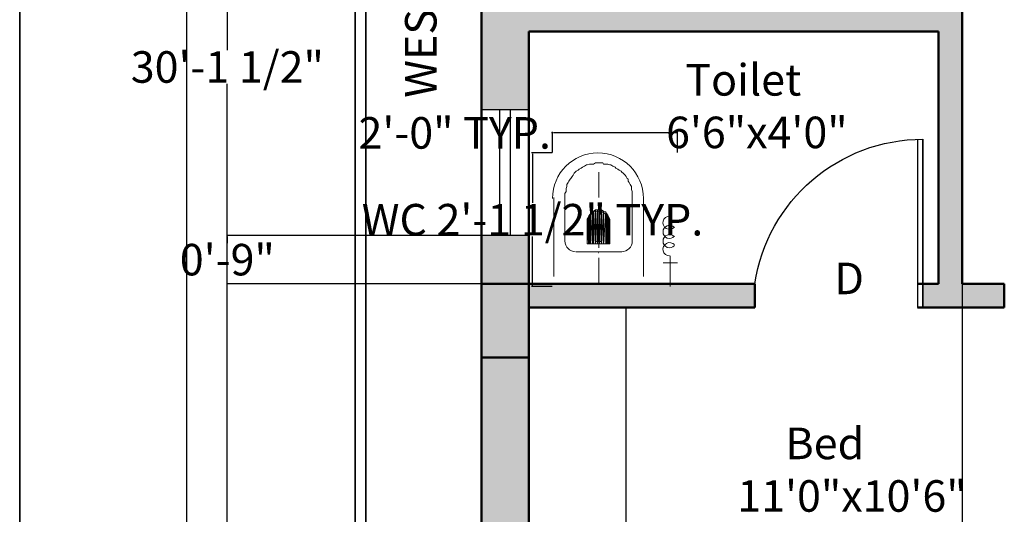
# Model space of a CAD drawing. Units: inches. Extents: x 1601 to 2080, y 5000 to 5589.
# Tile 2 of 11: x 1601 to 1788, y 5165 to 5259. Entities that reach past the tile are written whole.
import ezdxf

# ---------------------------------------------------------------- set-up
doc = ezdxf.new("R2010")
doc.units = ezdxf.units.IN
doc.header["$MEASUREMENT"] = 0
for name, color, linetype, lineweight in [('A-ANNO-DIMS', 2, 'Continuous', 18), ('A-ANNO-TEXT', 7, 'Continuous', 25), ('A-ANNO-TTLB', 7, 'Continuous', 35), ('A-AREA-IDEN', 7, 'Continuous', 25), ('A-COLS', 7, 'Continuous', 50), ('A-COLS-PATT', 18, 'Continuous', 13), ('A-DOOR', 3, 'Continuous', 25), ('A-FLOR-CASE', 8, 'Continuous', 25), ('A-FLOR-FIXT', 7, 'Continuous', 18), ('A-GLAZ', 4, 'Continuous', 25), ('A-WALL', 7, 'Continuous', 50), ('A-WALL-PATT', 241, 'Continuous', 13), ('C-PROP', 7, 'Continuous', 35)]:
    doc.layers.add(name, color=color, linetype=linetype, lineweight=lineweight)
doc.styles.get("Standard").update_dxf_attribs({"font": 'arial.ttf'})
doc.dimstyles.get("Standard").update_dxf_attribs({"dimtxt": 6, "dimasz": 0.18, "dimexe": 0.18, "dimexo": 0.0625, "dimgap": 0.09, "dimtad": 0, "dimtih": 1, "dimtoh": 1, "dimdec": 1, "dimzin": 0, "dimdsep": 46, "dimlunit": 3, "dimtxsty": 'Standard', "dimcen": 0.09, "dimadec": 0, "dimazin": 0, "dimtfac": 1, "dimtdec": 1, "dimtofl": 0, "dimtmove": 0, "dimatfit": 3, "dimfxl": 1, "dimtolj": 1, "dimtzin": 0, "dimarcsym": 0})

# ---------------------------------------------------------------- blocks, each defined once
blk = doc.blocks.new('*D4')
at = {"layer": 'A-ANNO-DIMS', "color": 0, "lineweight": -2, "transparency": 16777216}
for p, q in [((1664.35, 5509.2), (1632.18, 5509.2)), ((1632.36, 5509.02), (1632.36, 5281.35)), ((1632.36, 5047.39), (1632.36, 5275.05)), ((1664.35, 5047.21), (1632.18, 5047.21))]:
    blk.add_line(p, q, dxfattribs=at)
at = {"layer": 'A-ANNO-DIMS', "color": 0, "transparency": 16777216}
for points in [[(1632.33, 5509.02), (1632.39, 5509.02), (1632.36, 5509.2)], [(1632.33, 5047.39), (1632.39, 5047.39), (1632.36, 5047.21)]]:
    blk.add_solid(points, dxfattribs=at)
at = {"layer": 'Defpoints', "color": 0, "transparency": 16777216}
for p in [(1664.41, 5509.2), (1632.36, 5047.21), (1664.41, 5047.21)]:
    blk.add_point(p, dxfattribs=at)
at = {"layer": 'A-ANNO-DIMS', "color": 0, "transparency": 16777216, "insert": (1632.36, 5278.2), "char_height": 6, "attachment_point": 5}
blk.add_mtext("\\A1;40'", dxfattribs=at)
blk = doc.blocks.new('WC')
h = blk.add_hatch(color=256)
h.paths.add_polyline_path([(12.84, 17.3), (12.84, 12.59), (13.07, 17.3)])
h.paths.add_polyline_path([(12.84, 12.59), (13.07, 17.3), (13.07, 12.21)])
h = blk.add_hatch(color=256)
h.paths.add_polyline_path([(13.07, 17.3), (13.07, 12.21), (13.22, 17.3)])
h.paths.add_polyline_path([(13.07, 12.21), (13.22, 17.3), (13.22, 11.83)])
h = blk.add_hatch(color=256)
h.paths.add_polyline_path([(13.22, 17.3), (13.22, 11.83), (13.45, 17.3)])
h.paths.add_polyline_path([(13.22, 11.83), (13.45, 17.3), (13.45, 11.61)])
h = blk.add_hatch(color=256)
h.paths.add_polyline_path([(13.45, 17.3), (13.45, 11.61), (13.6, 17.3)])
h.paths.add_polyline_path([(13.45, 11.61), (13.6, 17.3), (13.6, 11.23)])
h = blk.add_hatch(color=256)
h.paths.add_polyline_path([(13.6, 17.3), (13.6, 11.23), (14.06, 17.3)])
h.paths.add_polyline_path([(13.6, 11.23), (14.06, 17.3), (14.06, 11.08)])
h = blk.add_hatch(color=256)
h.paths.add_polyline_path([(14.06, 17.3), (14.06, 11.08), (14.44, 17.3)])
h.paths.add_polyline_path([(14.06, 11.08), (14.44, 17.3), (14.44, 10.85)])
h = blk.add_hatch(color=256)
h.paths.add_polyline_path([(14.44, 17.3), (14.44, 10.85), (14.81, 17.3)])
h.paths.add_polyline_path([(14.44, 10.85), (14.81, 17.3), (14.81, 10.85)])
h = blk.add_hatch(color=256)
h.paths.add_polyline_path([(14.81, 17.3), (14.81, 10.85), (15.19, 17.3)])
h.paths.add_polyline_path([(14.81, 10.85), (15.19, 17.3), (15.19, 10.85)])
h = blk.add_hatch(color=256)
h.paths.add_polyline_path([(15.19, 17.3), (15.19, 10.85), (15.57, 17.3)])
h.paths.add_polyline_path([(15.19, 10.85), (15.57, 17.3), (15.57, 10.85)])
h = blk.add_hatch(color=256)
h.paths.add_polyline_path([(15.57, 17.3), (15.57, 10.85), (15.95, 17.3)])
h.paths.add_polyline_path([(15.57, 10.85), (15.95, 17.3), (15.95, 11.08)])
h = blk.add_hatch(color=256)
h.paths.add_polyline_path([(15.95, 17.3), (15.95, 11.08), (16.18, 17.3)])
h.paths.add_polyline_path([(15.95, 11.08), (16.18, 17.3), (16.18, 11.23)])
h = blk.add_hatch(color=256)
h.paths.add_polyline_path([(16.18, 17.3), (16.18, 11.23), (16.56, 17.3)])
h.paths.add_polyline_path([(16.18, 11.23), (16.56, 17.3), (16.56, 11.61)])
h = blk.add_hatch(color=256)
h.paths.add_polyline_path([(16.56, 17.3), (16.56, 11.61), (16.71, 17.3)])
h.paths.add_polyline_path([(16.56, 11.61), (16.71, 17.3), (16.71, 11.83)])
h = blk.add_hatch(color=256)
h.paths.add_polyline_path([(16.71, 17.3), (16.71, 11.83), (16.94, 17.3)])
h.paths.add_polyline_path([(16.71, 11.83), (16.94, 17.3), (16.94, 12.21)])
h = blk.add_hatch(color=256)
h.paths.add_polyline_path([(16.94, 17.3), (16.94, 12.21), (17.17, 17.3)])
h.paths.add_polyline_path([(16.94, 12.21), (17.17, 17.3), (17.17, 12.59)])
h.paths.add_polyline_path([(17.17, 17.3), (17.17, 12.59), (17.17, 12.97)])
for points in [[(1.37, 25.41), (1.37, 19.57), (1.37, 19.57)], [(14.97, 24.81), (14.97, 19.95), (14.97, 19.95)], [(6.47, 23.52), (6.47, 8.5), (6.47, 8.5)], [(23.54, 23.52), (23.54, 8.5), (23.54, 8.5)], [(2.73, 20.94), (0, 20.94), (0, 20.94)], [(19.29, 18.81), (10.57, 18.81), (10.57, 18.81)], [(14.97, 19.04), (15.04, 19.04), (15.04, 19.04)], [(17.17, 17.3), (12.84, 17.3), (12.84, 17.3)], [(12.84, 17.3), (12.84, 12.97), (12.84, 12.97)], [(14.59, 16.84), (14.59, 16.92), (14.59, 16.92)], [(14.97, 18.05), (14.97, 10.47), (14.97, 10.47)], [(14.97, 16.84), (15.04, 16.92), (15.04, 16.92)], [(15.42, 16.84), (15.42, 16.92), (15.42, 16.92)], [(17.17, 17.3), (17.17, 12.97), (17.17, 12.97)], [(8.59, 16.69), (8.59, 9.48), (8.59, 9.48)], [(14.97, 16.84), (14.81, 16.84), (14.59, 16.84)], [(15.42, 16.84), (15.19, 16.84), (14.97, 16.84)], [(21.41, 16.69), (21.41, 9.48), (21.41, 9.48)], [(21.41, 9.48), (21.41, 8.72), (21.41, 8.12), (21.41, 7.74), (21.19, 7.36), (21.19, 6.98), (21.19, 6.75), (21.03, 6.37), (21.03, 5.99), (20.81, 5.61), (20.66, 5.39), (20.43, 5.01), (20.28, 4.85), (20.05, 4.48), (19.82, 4.25), (19.67, 3.87), (19.44, 3.64), (19.29, 3.49), (18.91, 3.26), (18.68, 3.11), (18.3, 2.88), (18.08, 2.73), (17.7, 2.5), (17.32, 2.28), (17.17, 2.28), (16.71, 2.12), (16.33, 2.12), (15.95, 2.12), (15.57, 1.9), (14.97, 1.9), (14.21, 1.9), (14.06, 2.12), (13.6, 2.12), (13.22, 2.12), (12.84, 2.28), (12.69, 2.28), (12.31, 2.5), (11.86, 2.73), (11.7, 2.88), (11.32, 3.11), (11.1, 3.26), (10.72, 3.49), (10.57, 3.64), (10.34, 3.87), (9.96, 4.25), (9.73, 4.48), (9.58, 4.85), (9.35, 5.01), (9.35, 5.39), (9.2, 5.61), (8.97, 5.99), (8.75, 6.37), (8.75, 6.75), (8.75, 6.98), (8.59, 7.36), (8.59, 7.74), (8.59, 8.12), (8.59, 8.72), (8.59, 9.48)], [(14.97, 8.5), (14.97, 3.64), (14.97, 3.64)]]:
    blk.add_lwpolyline(points)
for points in [[(12.84, 17.3), (12.84, 12.97)], [(12.84, 12.97), (12.84, 17.3), (12.84, 12.59)], [(12.84, 17.3), (12.84, 12.59), (13.07, 17.3)], [(12.84, 12.59), (13.07, 17.3), (13.07, 12.21)], [(13.07, 17.3), (13.07, 12.21), (13.22, 17.3)], [(13.07, 12.21), (13.22, 17.3), (13.22, 11.83)], [(13.22, 17.3), (13.22, 11.83), (13.45, 17.3)], [(13.22, 11.83), (13.45, 17.3), (13.45, 11.61)], [(13.45, 17.3), (13.45, 11.61), (13.6, 17.3)], [(13.45, 11.61), (13.6, 17.3), (13.6, 11.23)], [(13.6, 17.3), (13.6, 11.23), (14.06, 17.3)], [(13.6, 11.23), (14.06, 17.3), (14.06, 11.08)], [(14.06, 17.3), (14.06, 11.08), (14.44, 17.3)], [(14.06, 11.08), (14.44, 17.3), (14.44, 10.85)], [(14.44, 17.3), (14.44, 10.85), (14.81, 17.3)], [(14.44, 10.85), (14.81, 17.3), (14.81, 10.85)], [(14.81, 17.3), (14.81, 10.85), (15.19, 17.3)], [(14.81, 10.85), (15.19, 17.3), (15.19, 10.85)], [(15.19, 17.3), (15.19, 10.85), (15.57, 17.3)], [(15.19, 10.85), (15.57, 17.3), (15.57, 10.85)], [(15.57, 17.3), (15.57, 10.85), (15.95, 17.3)], [(15.57, 10.85), (15.95, 17.3), (15.95, 11.08)], [(15.95, 17.3), (15.95, 11.08), (16.18, 17.3)], [(15.95, 11.08), (16.18, 17.3), (16.18, 11.23)], [(16.18, 17.3), (16.18, 11.23), (16.56, 17.3)], [(16.18, 11.23), (16.56, 17.3), (16.56, 11.61)], [(16.56, 17.3), (16.56, 11.61), (16.71, 17.3)], [(16.56, 11.61), (16.71, 17.3), (16.71, 11.83)], [(16.71, 17.3), (16.71, 11.83), (16.94, 17.3)], [(16.71, 11.83), (16.94, 17.3), (16.94, 12.21)], [(16.94, 17.3), (16.94, 12.21), (17.17, 17.3)], [(16.94, 12.21), (17.17, 17.3), (17.17, 12.59)], [(17.17, 17.3), (17.17, 12.59), (17.17, 12.97)], [(17.17, 12.59), (17.17, 17.3), (17.17, 17.3)]]:
    blk.add_lwpolyline(points, close=True)
for points, knots in [([(0.53, 17.45), (0.91, 17.07), (1.59, 16.92), (2.05, 17.22), (2.05, 17.22), (2.58, 17.52), (2.88, 18.05), (2.73, 18.66), (2.73, 18.66), (2.58, 19.19), (2.05, 19.57), (1.52, 19.57)], [0, 0, 0, 0, 0.083333, 0.083333, 0.083333, 0.083334, 0.166667, 0.166667, 0.166667, 0.166668, 1, 1, 1, 1]), ([(0.61, 15.93), (0.91, 15.55), (1.52, 15.4), (1.97, 15.63), (1.97, 15.63), (2.43, 15.78), (2.73, 16.31), (2.73, 16.76), (2.73, 16.76), (2.73, 17.3), (2.43, 17.75), (1.97, 17.98), (1.97, 17.98), (1.44, 18.13), (0.91, 17.98), (0.53, 17.6)], [0, 0, 0, 0, 0.0625, 0.0625, 0.0625, 0.062501, 0.125, 0.125, 0.125, 0.125001, 0.1875, 0.1875, 0.1875, 0.187501, 1, 1, 1, 1]), ([(0.53, 14.19), (0.91, 13.81), (1.44, 13.65), (1.97, 13.88), (1.97, 13.88), (2.43, 14.03), (2.73, 14.49), (2.73, 15.02), (2.73, 15.02), (2.73, 15.55), (2.43, 16.01), (1.97, 16.23), (1.97, 16.23), (1.44, 16.39), (0.91, 16.23), (0.53, 15.85)], [0, 0, 0, 0, 0.0625, 0.0625, 0.0625, 0.062501, 0.125, 0.125, 0.125, 0.125001, 0.1875, 0.1875, 0.1875, 0.187501, 1, 1, 1, 1]), ([(1.52, 11.99), (2.05, 11.99), (2.58, 12.44), (2.73, 12.97), (2.73, 12.97), (2.88, 13.5), (2.58, 14.11), (2.12, 14.41), (2.12, 14.41), (1.59, 14.64), (0.99, 14.56), (0.61, 14.19)], [0, 0, 0, 0, 0.083333, 0.083333, 0.083333, 0.083334, 0.166667, 0.166667, 0.166667, 0.166668, 1, 1, 1, 1]), ([(13.07, 13.12), (13.07, 11.99), (13.98, 11.08), (15.12, 11.08), (15.12, 11.08), (16.26, 11.08), (17.17, 11.99), (17.17, 13.12)], [0, 0, 0, 0, 0.125, 0.125, 0.125, 0.125001, 1, 1, 1, 1]), ([(6.47, 8.65), (6.47, 3.87), (10.34, 0), (15.12, 0), (15.12, 0), (19.9, 0), (23.77, 3.87), (23.77, 8.65)], [0, 0, 0, 0, 0.125, 0.125, 0.125, 0.125001, 1, 1, 1, 1])]:
    blk.add_open_spline(points, degree=3, knots=knots)
for points in [[(10.64, 18.81), (9.5, 18.81), (8.59, 17.9), (8.59, 16.76)], [(21.41, 16.76), (21.41, 17.9), (20.5, 18.81), (19.37, 18.81)]]:
    blk.add_open_spline(points, degree=3)
blk = doc.blocks.new('DOOR-32IN')
for p, q in [((32, 32), (31, 32)), ((31, 0), (31, 32)), ((32, 32), (32, 0)), ((32, 0), (32, 32))]:
    blk.add_line(p, q)
blk.add_arc((32, 32.37), 32.37, 188.6501, 270)
blk = doc.blocks.new('VENT-24IN')
for p, q in [((0, 0), (0, 24)), ((0, 24), (9, 24)), ((3.5, 0), (3.5, 24)), ((5.5, 24), (5.5, 0)), ((9, 24), (9, 0)), ((9, 0), (0, 0))]:
    blk.add_line(p, q)
blk = doc.blocks.new('*D21')
at = {"layer": 'A-ANNO-DIMS', "color": 0, "lineweight": -2, "transparency": 16777216}
for p, q in [((1701.88, 5234.1), (1697.95, 5234.1)), ((1698.13, 5233.92), (1698.13, 5224.58)), ((1698.13, 5208.87), (1698.13, 5218.2)), ((1701.88, 5208.69), (1697.95, 5208.69))]:
    blk.add_line(p, q, dxfattribs=at)
at = {"layer": 'A-ANNO-DIMS', "color": 0, "transparency": 16777216}
for points in [[(1698.1, 5233.92), (1698.16, 5233.92), (1698.13, 5234.1)], [(1698.1, 5208.87), (1698.16, 5208.87), (1698.13, 5208.69)]]:
    blk.add_solid(points, dxfattribs=at)
at = {"layer": 'Defpoints', "color": 0, "transparency": 16777216}
for p in [(1701.94, 5234.1), (1698.13, 5208.69), (1701.94, 5208.69)]:
    blk.add_point(p, dxfattribs=at)
at = {"layer": 'A-ANNO-DIMS', "color": 0, "transparency": 16777216, "insert": (1698.13, 5221.39), "char_height": 6, "attachment_point": 5}
blk.add_mtext('\\A1;WC 2\'-1 1/2" TYP.', dxfattribs=at)
blk = doc.blocks.new('*D22')
at = {"layer": 'A-ANNO-DIMS', "color": 0, "lineweight": -2, "transparency": 16777216}
for p, q in [((1701.94, 5237.91), (1701.76, 5237.91)), ((1701.94, 5234.16), (1701.94, 5238.09)), ((1725.52, 5237.91), (1702.12, 5237.91)), ((1725.7, 5234.16), (1725.7, 5238.09))]:
    blk.add_line(p, q, dxfattribs=at)
at = {"layer": 'A-ANNO-DIMS', "color": 0, "transparency": 16777216}
for points in [[(1702.12, 5237.94), (1702.12, 5237.88), (1701.94, 5237.91)], [(1725.52, 5237.94), (1725.52, 5237.88), (1725.7, 5237.91)]]:
    blk.add_solid(points, dxfattribs=at)
at = {"layer": 'Defpoints', "color": 0, "transparency": 16777216}
for p in [(1701.94, 5237.91), (1701.94, 5234.1), (1725.7, 5234.1)]:
    blk.add_point(p, dxfattribs=at)
at = {"layer": 'A-ANNO-DIMS', "color": 0, "transparency": 16777216, "insert": (1683.33, 5237.91), "char_height": 6, "attachment_point": 5}
blk.add_mtext('\\A1;2\'-0" TYP.', dxfattribs=at)
blk = doc.blocks.new('*D38')
at = {"layer": 'A-ANNO-DIMS', "color": 0, "lineweight": -2, "transparency": 16777216}
for p, q in [((1688.35, 5431.2), (1639.88, 5431.2)), ((1640.06, 5431.02), (1640.06, 5253.64)), ((1640.06, 5069.88), (1640.06, 5247.25)), ((1688.35, 5069.7), (1639.88, 5069.7))]:
    blk.add_line(p, q, dxfattribs=at)
at = {"layer": 'A-ANNO-DIMS', "color": 0, "transparency": 16777216}
for points in [[(1640.03, 5431.02), (1640.09, 5431.02), (1640.06, 5431.2)], [(1640.03, 5069.88), (1640.09, 5069.88), (1640.06, 5069.7)]]:
    blk.add_solid(points, dxfattribs=at)
at = {"layer": 'Defpoints', "color": 0, "transparency": 16777216}
for p in [(1640.06, 5431.2), (1688.41, 5431.2), (1688.41, 5069.7)]:
    blk.add_point(p, dxfattribs=at)
at = {"layer": 'A-ANNO-DIMS', "color": 0, "transparency": 16777216, "insert": (1640.06, 5250.45), "char_height": 6, "attachment_point": 5}
blk.add_mtext('\\A1;30\'-1 1/2"', dxfattribs=at)
blk = doc.blocks.new('*D52')
at = {"layer": 'A-ANNO-DIMS', "color": 0, "lineweight": -2, "transparency": 16777216}
for p, q in [((1688.35, 5218.37), (1639.88, 5218.37)), ((1640.06, 5218.19), (1640.06, 5216.94)), ((1640.06, 5209.38), (1640.06, 5210.63)), ((1688.35, 5209.2), (1639.88, 5209.2))]:
    blk.add_line(p, q, dxfattribs=at)
at = {"layer": 'A-ANNO-DIMS', "color": 0, "transparency": 16777216}
for points in [[(1640.03, 5218.19), (1640.09, 5218.19), (1640.06, 5218.37)], [(1640.03, 5209.38), (1640.09, 5209.38), (1640.06, 5209.2)]]:
    blk.add_solid(points, dxfattribs=at)
at = {"layer": 'Defpoints', "color": 0, "transparency": 16777216}
for p in [(1640.06, 5218.37), (1688.41, 5218.37), (1688.41, 5209.2)]:
    blk.add_point(p, dxfattribs=at)
at = {"layer": 'A-ANNO-DIMS', "color": 0, "transparency": 16777216, "insert": (1640.06, 5213.79), "char_height": 6, "attachment_point": 5}
blk.add_mtext('\\A1;0\'-9"', dxfattribs=at)
blk = doc.blocks.new('*D58')
at = {"layer": 'A-ANNO-DIMS', "color": 0, "lineweight": -2, "transparency": 16777216}
for p, q in [((1779.91, 5209.13), (1779.91, 5022.68)), ((1824.91, 5209.13), (1824.91, 5022.68)), ((1780.09, 5022.86), (1794.35, 5022.86)), ((1824.73, 5022.86), (1810.47, 5022.86))]:
    blk.add_line(p, q, dxfattribs=at)
at = {"layer": 'A-ANNO-DIMS', "color": 0, "transparency": 16777216}
for points in [[(1780.09, 5022.89), (1780.09, 5022.83), (1779.91, 5022.86)], [(1824.73, 5022.89), (1824.73, 5022.83), (1824.91, 5022.86)]]:
    blk.add_solid(points, dxfattribs=at)
at = {"layer": 'Defpoints', "color": 0, "transparency": 16777216}
for p in [(1779.91, 5209.2), (1824.91, 5209.2), (1824.91, 5022.86)]:
    blk.add_point(p, dxfattribs=at)
at = {"layer": 'A-ANNO-DIMS', "color": 0, "transparency": 16777216, "insert": (1802.41, 5022.86), "char_height": 6, "attachment_point": 5}
blk.add_mtext('\\A1;3\'-9"', dxfattribs=at)

msp = doc.modelspace()

# ---------------------------------------------------------------- hatches: boundary and pattern name
at = {"layer": 'A-COLS-PATT'}
h = msp.add_hatch(color=256, dxfattribs=at)
h.dxf.hatch_style = 1
h.paths.add_polyline_path([(1702.41, 5431.2), (1688.41, 5431.2), (1688.41, 5422.2), (1702.41, 5422.2)])
h.paths.add_polyline_path([(1836.17, 5431.2), (1822.17, 5431.2), (1822.17, 5422.2), (1836.17, 5422.2)])
h.paths.add_polyline_path([(1962.91, 5431.2), (1948.91, 5431.2), (1948.91, 5422.2), (1962.91, 5422.2)])
h.paths.add_polyline_path([(1697.41, 5314.2), (1688.41, 5314.2), (1688.41, 5300.2), (1697.41, 5300.2)])
h.paths.add_polyline_path([(1833.91, 5314.2), (1824.91, 5314.2), (1824.91, 5300.2), (1833.91, 5300.2)])
h.paths.add_polyline_path([(1962.91, 5314.2), (1953.91, 5314.2), (1953.91, 5300.2), (1962.91, 5300.2)])
h.paths.add_polyline_path([(1697.41, 5209.2), (1688.41, 5209.2), (1688.41, 5195.2), (1697.41, 5195.2)])
h.paths.add_polyline_path([(1833.91, 5209.2), (1824.91, 5209.2), (1824.91, 5195.2), (1833.91, 5195.2)])
h.paths.add_polyline_path([(1962.91, 5209.2), (1953.91, 5209.2), (1953.91, 5195.2), (1962.91, 5195.2)])
h.paths.add_polyline_path([(1697.41, 5083.7), (1688.41, 5083.7), (1688.41, 5069.7), (1697.41, 5069.7)])
h.paths.add_polyline_path([(1833.91, 5078.7), (1819.91, 5078.7), (1819.91, 5069.7), (1833.91, 5069.7)])
h.paths.add_polyline_path([(1962.91, 5078.7), (1948.91, 5078.7), (1948.91, 5069.7), (1962.91, 5069.7)])
at = {"layer": 'A-WALL-PATT'}
h = msp.add_hatch(color=256, dxfattribs=at)
h.dxf.hatch_style = 1
h.paths.add_polyline_path([(1763.95, 5431.2), (1702.41, 5431.2), (1702.41, 5422.2), (1763.95, 5422.2)])
h.paths.add_polyline_path([(1697.41, 5422.2), (1688.41, 5422.2), (1688.41, 5314.2), (1697.41, 5314.2)])
h.paths.add_polyline_path([(1740.41, 5314.2), (1697.41, 5314.2), (1697.41, 5309.7), (1740.41, 5309.7)], flags=17)
h.paths.add_polyline_path([(1822.17, 5431.2), (1811.95, 5431.2), (1811.95, 5422.2), (1822.17, 5422.2)])
h.paths.add_polyline_path([(1845.52, 5431.2), (1836.17, 5431.2), (1836.17, 5422.2), (1845.52, 5422.2)])
h.paths.add_polyline_path([(1910.91, 5431.2), (1881.52, 5431.2), (1881.52, 5422.2), (1910.91, 5422.2)])
h.paths.add_polyline_path([(1948.91, 5431.2), (1945.91, 5431.2), (1942.91, 5431.2), (1942.91, 5422.2), (1948.91, 5422.2)])
h.paths.add_polyline_path([(1962.91, 5422.2), (1953.91, 5422.2), (1953.91, 5416.29), (1962.91, 5416.29)])
h.paths.add_polyline_path([(1962.91, 5384.29), (1953.91, 5384.29), (1953.91, 5381.29), (1962.91, 5381.29)])
h.paths.add_polyline_path([(1962.91, 5333.29), (1953.91, 5333.29), (1953.91, 5314.2), (1962.91, 5314.2)])
h.paths.add_polyline_path([(1962.91, 5300.2), (1953.91, 5300.2), (1953.91, 5236.2), (1875.91, 5236.2), (1875.91, 5230.7), (1881.91, 5230.7), (1881.91, 5231.7), (1953.91, 5231.7), (1953.91, 5219.2), (1962.91, 5219.2)])
h.paths.add_polyline_path([(1962.91, 5185.2), (1953.91, 5185.2), (1953.91, 5183.7), (1881.91, 5183.7), (1881.91, 5184.7), (1875.91, 5184.7), (1875.91, 5183.7), (1875.91, 5179.2), (1953.91, 5179.2), (1953.91, 5172.6), (1962.91, 5172.6)])
h.paths.add_polyline_path([(1962.91, 5136.6), (1953.91, 5136.6), (1953.91, 5078.7), (1962.91, 5078.7)])
h.paths.add_polyline_path([(1948.91, 5078.7), (1833.91, 5078.7), (1833.91, 5069.7), (1948.91, 5069.7)])
h.paths.add_polyline_path([(1833.91, 5195.2), (1829.41, 5195.2), (1829.41, 5078.7), (1833.91, 5078.7)])
h.paths.add_polyline_path([(1819.91, 5078.7), (1813.58, 5078.7), (1813.58, 5069.7), (1819.91, 5069.7)])
h.paths.add_polyline_path([(1765.58, 5078.7), (1697.41, 5078.7), (1697.41, 5069.7), (1765.58, 5069.7)])
h.paths.add_polyline_path([(1697.41, 5195.2), (1688.41, 5195.2), (1688.41, 5083.7), (1697.41, 5083.7)])
h.paths.add_polyline_path([(1740.41, 5209.2), (1697.41, 5209.2), (1697.41, 5204.7), (1740.41, 5204.7)], flags=17)
h.paths.add_polyline_path([(1787.91, 5209.2), (1779.91, 5209.2), (1779.91, 5309.7), (1787.91, 5309.7), (1787.91, 5314.2), (1772.41, 5314.2), (1772.41, 5309.7), (1775.41, 5309.7), (1775.41, 5261.7), (1697.41, 5261.7), (1697.41, 5273.07), (1688.41, 5273.07), (1688.41, 5242.37), (1697.41, 5242.37), (1697.41, 5257.2), (1775.41, 5257.2), (1775.41, 5209.2), (1772.41, 5209.2), (1772.41, 5204.7), (1775.41, 5204.7), (1787.91, 5204.7)])
h.paths.add_polyline_path([(1697.41, 5218.37), (1688.41, 5218.37), (1688.41, 5209.2), (1697.41, 5209.2)], flags=17)
h.paths.add_polyline_path([(1833.91, 5422.2), (1829.41, 5422.2), (1829.41, 5314.2), (1833.91, 5314.2)])
h.paths.add_polyline_path([(1697.41, 5300.2), (1688.41, 5300.2), (1688.41, 5297.07), (1697.41, 5297.07)], flags=17)

# ---------------------------------------------------------------- linework, layer by layer
at = {"layer": 'A-ANNO-TTLB'}
msp.add_lwpolyline([(1600.55, 5589.45), (2079.72, 5589.45), (2079.72, 4999.95), (1600.55, 4999.95)], close=True, dxfattribs=at)
at = {"layer": 'A-COLS'}
for p, q in [((1688.41, 5209.2), (1688.41, 5195.2)), ((1697.41, 5195.2), (1697.41, 5209.2)), ((1688.41, 5195.2), (1697.41, 5195.2))]:
    msp.add_line(p, q, dxfattribs=at)
at = {"layer": 'A-FLOR-CASE'}
msp.add_line((1715.89, 5204.7), (1715.89, 5078.7), dxfattribs=at)
at = {"layer": 'A-WALL'}
for p, q in [((1688.41, 5431.2), (1688.41, 5069.7)), ((1779.91, 5309.7), (1779.91, 5209.2)), ((1697.41, 5257.2), (1775.41, 5257.2)), ((1697.41, 5257.2), (1697.41, 5069.7)), ((1775.41, 5257.2), (1775.41, 5209.2)), ((1688.41, 5209.2), (1740.41, 5209.2)), ((1740.41, 5204.7), (1740.41, 5209.2)), ((1771.41, 5209.2), (1775.41, 5209.2)), ((1779.91, 5209.2), (1787.91, 5209.2)), ((1787.91, 5209.2), (1787.91, 5204.7)), ((1697.41, 5204.7), (1740.41, 5204.7)), ((1771.41, 5204.7), (1787.91, 5204.7)), ((1775.41, 5204.7), (1772.41, 5204.7))]:
    msp.add_line(p, q, dxfattribs=at)
at = {"layer": 'C-PROP'}
for p, q in [((1664.41, 5509.2), (1664.41, 5047.21)), ((1666.41, 5507.2), (1666.41, 5069.7))]:
    msp.add_line(p, q, dxfattribs=at)

# ---------------------------------------------------------------- block references
at = {"layer": 'A-DOOR', "extrusion": (0, 0, -1), "zscale": -1, "rotation": 180}
msp.add_blockref('DOOR-32IN', (-1740.41, 5236.7), dxfattribs=at)
at = {"layer": 'A-FLOR-FIXT', "rotation": 180}
msp.add_blockref('WC', (1725.7, 5234.1), dxfattribs=at)
at = {"layer": 'A-GLAZ'}
msp.add_blockref('VENT-24IN', (1688.41, 5218.37), dxfattribs=at)

# ---------------------------------------------------------------- texts
at = {"layer": 'A-ANNO-TEXT', "insert": (1755.57, 5213.22), "char_height": 6, "attachment_point": 1}
msp.add_mtext_dynamic_manual_height_columns('D ', width=9.7695, gutter_width=30, heights=[0], dxfattribs=at)
at = {"layer": 'A-AREA-IDEN', "insert": (1673.87, 5244.59), "char_height": 6, "attachment_point": 1, "rotation": 90}
msp.add_mtext_dynamic_manual_height_columns("WEST OPEN SPACE - 2'", width=126.5515, gutter_width=30, heights=[0], dxfattribs=at)
at = {"layer": 'A-AREA-IDEN', "char_height": 6, "attachment_point": 1}
for s, width, insert in [('  Toilet\\P6\'6"x4\'0"', 35.0416, (1723.54, 5251)), ('     Bed\\P11\'0"x10\'6"', 52.5217, (1737.1, 5181.83))]:
    msp.add_mtext_dynamic_manual_height_columns(s, width=width, gutter_width=30, heights=[0], dxfattribs=dict(at, insert=insert))

# ---------------------------------------------------------------- dimensions: what is measured, and where the dimension line sits
at = {"layer": 'A-ANNO-DIMS'}
for base, p1, p2, angle, text, override, picture, middle in [((1632.36, 5047.21), (1664.41, 5509.2), (1664.41, 5047.21), 90, "40'", {"dimclrd": 0, "dimclre": 0, "dimclrt": 0}, '*D4', (1632.36, 5278.2)), ((1701.94, 5237.91), (1725.7, 5234.1), (1701.94, 5234.1), 180, '<> TYP.', {"dimdec": 1, "dimlfac": 1, "dimrnd": 0, "dimzin": 1, "dimdsep": 46, "dimlunit": 4, "dimfrac": 2}, '*D22', (1683.33, 5237.91)), ((1698.13, 5208.69), (1701.94, 5234.1), (1701.94, 5208.69), 270, 'WC <> TYP.', {"dimdec": 1, "dimlfac": 1, "dimrnd": 0, "dimzin": 1, "dimdsep": 46, "dimlunit": 4, "dimfrac": 2}, '*D21', (1698.13, 5221.39))]:
    dim = msp.add_linear_dim(base=base, p1=p1, p2=p2, angle=angle, text=text, dimstyle='Standard', override=override, dxfattribs=at)
    dim.commit()
    dim.dimension.update_dxf_attribs({"geometry": picture, "text_midpoint": middle})
for base, p1, p2, picture, middle in [((1640.06, 5431.2), (1688.41, 5069.7), (1688.41, 5431.2), '*D38', (1640.06, 5250.45)), ((1640.06, 5218.37), (1688.41, 5209.2), (1688.41, 5218.37), '*D52', (1640.06, 5213.79))]:
    dim = msp.add_linear_dim(base=base, p1=p1, p2=p2, angle=90, dimstyle='Standard', override={"dimdec": 1, "dimlfac": 1, "dimrnd": 0, "dimzin": 1, "dimdsep": 46, "dimlunit": 4, "dimfrac": 2}, dxfattribs=at)
    dim.commit()
    dim.dimension.update_dxf_attribs({"geometry": picture, "text_midpoint": middle})
dim = msp.add_linear_dim(base=(1824.91, 5022.86), p1=(1779.91, 5209.2), p2=(1824.91, 5209.2), dimstyle='Standard', override={"dimdec": 1, "dimlfac": 1, "dimrnd": 0, "dimzin": 1, "dimdsep": 46, "dimlunit": 4, "dimfrac": 2}, dxfattribs=at)
dim.commit()
dim.dimension.update_dxf_attribs({"geometry": '*D58', "text_midpoint": (1802.41, 5022.86)})

doc.saveas('drawing.dxf')
